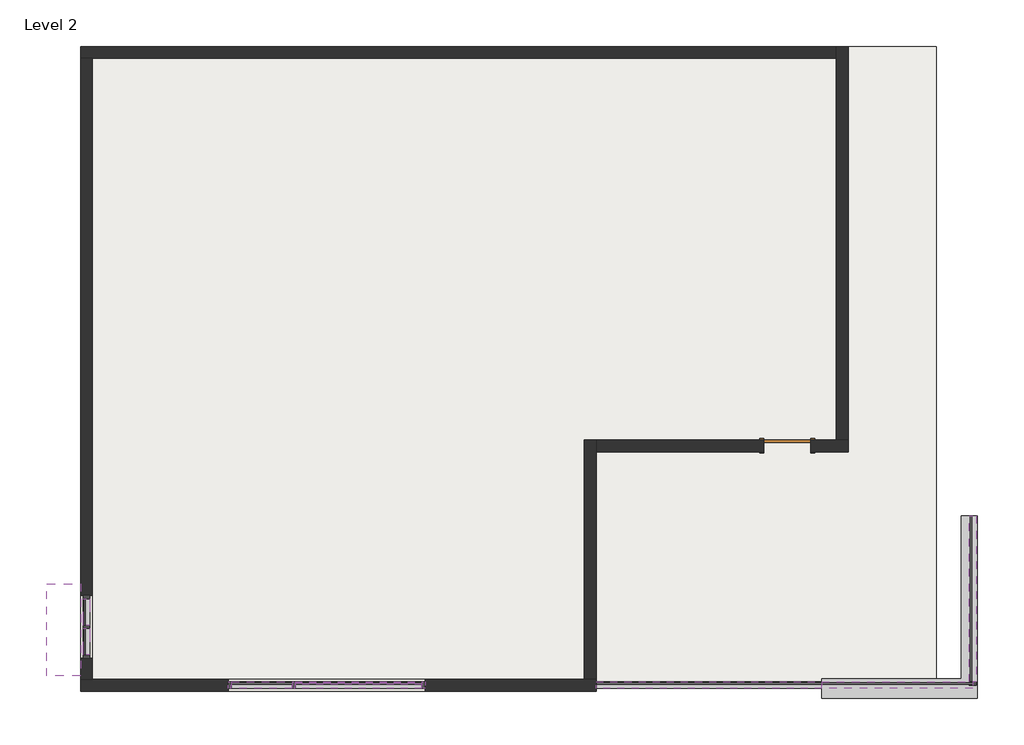
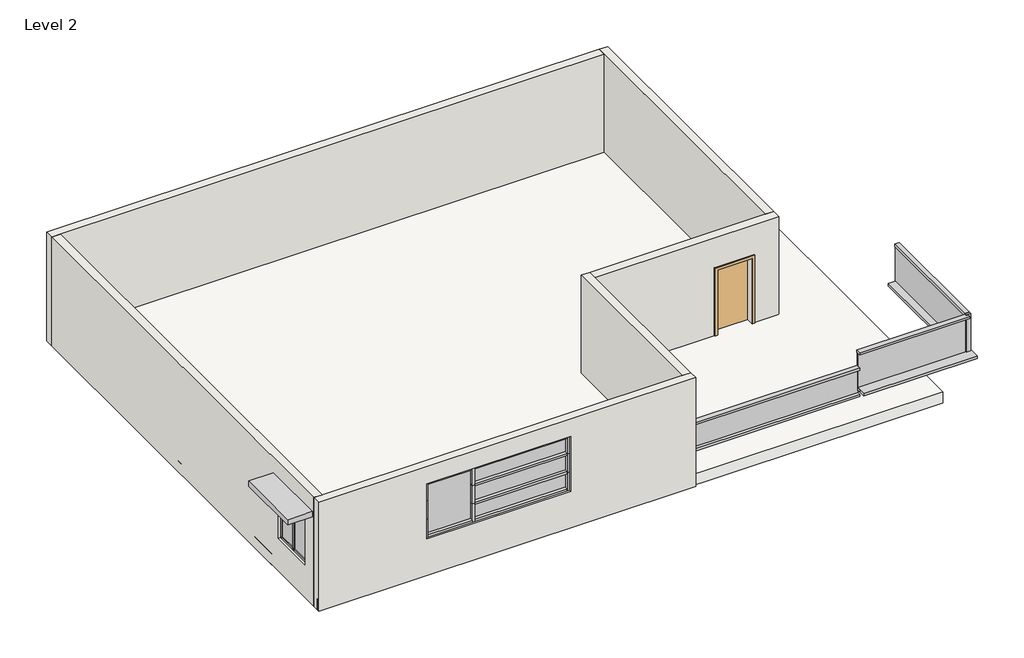
# One storey: 28 members, 9 plates, 6 walls, 2 proxies, 1 door, 1 roof.
"""IFC4 building model written with IfcOpenShell, lengths in millimetres."""

from ifc_helpers import new_model, si_unit, frame, origin, place, context, project, spatial, polyline, outline, extrude, faceted_brep, transform, mapped, element, save
from components import generic_models_3_generic_models_3_8d4ae4f9, generic_models_7_generic_models_7_15f6dc16, door_0ca8825f, member_794f270d, member_fb497cbf, member_38106158, member_c678549b, member_8e6e9988, member_0b7646a3, member_fff16b5b, member_15f14dc2, member_4a27761c, member_d457d5cf, member_01255749, member_1c5922cf, system_panel_glazed_93b0cd61, system_panel_glazed_07248474, system_panel_glazed_5c06d9ac, system_panel_glazed_cb7cf9ed, system_panel_glazed_bff90f26, system_panel_glazed_3fab1137, system_panel_glazed_82fe4a0c

model = new_model("IFC4")

# Units and contexts
model_context = context("Model", 3, world=origin())
ifc_project = project(units=[si_unit("LENGTHUNIT", "METRE", prefix="MILLI")], contexts=[model_context])

# Site, building, storey
site = spatial("IfcSite", under=ifc_project)
building = spatial("IfcBuilding", under=site)
storey = spatial("IfcBuildingStorey", under=building, Name="Level 2", Elevation=3048.0)

# Proxies
placement = place(None, origin())
generic_models_3_generic_models_3_shape = generic_models_3_generic_models_3_8d4ae4f9(model_context)
element("IfcBuildingElementProxy", 1, Name="Generic Models 3 : Generic Models 3", ObjectType="Generic Models 3 : Generic Models 3", at=placement, inside=storey, context=model_context, shape_type="MappedRepresentation", body=[
    mapped(generic_models_3_generic_models_3_shape, transform((0.0, 0.0, 0.0), x_axis=(1.0, 0.0, 0.0), y_axis=(0.0, 1.0, 0.0), z_axis=(0.0, 0.0, 1.0))),
])
generic_models_7_generic_models_7_shape = generic_models_7_generic_models_7_15f6dc16(model_context)
element("IfcBuildingElementProxy", 2, Name="Generic Models 7 : Generic Models 7", ObjectType="Generic Models 7 : Generic Models 7", at=placement, inside=storey, context=model_context, shape_type="MappedRepresentation", body=[
    mapped(generic_models_7_generic_models_7_shape, transform((0.0, 0.0, 0.0), x_axis=(1.0, 0.0, 0.0), y_axis=(0.0, 1.0, 0.0), z_axis=(0.0, 0.0, 1.0))),
])

# Door
door_shape = door_0ca8825f(model_context)
element("IfcDoor", 3, ObjectType="Single-Flush : 36\" x 84\"", at=placement, inside=storey, context=model_context, shape_type="MappedRepresentation", body=[
    mapped(door_shape, transform((-4164.5229687, -6103.4015118, 3048.0), x_axis=(1.0, 0.0, 0.0), y_axis=(0.0, 1.0, 0.0), z_axis=(0.0, 0.0, 1.0))),
])

# Members
member_shape = member_794f270d(model_context)
element("IfcMember", 4, ObjectType="Rectangular Mullion : 2.5\" x 5\" rectangular", at=placement, inside=storey, context=model_context, shape_type="MappedRepresentation", body=[
    mapped(member_shape, transform((-14984.9229687, -10738.9015118, 5099.2464705), x_axis=(-1.0, 0.0, 0.0), y_axis=(0.0, -1.0, 0.0), z_axis=(0.0, 0.0, 1.0))),
])
member_2_shape = member_fb497cbf(model_context)
element("IfcMember", 5, ObjectType="Rectangular Mullion : 2.5\" x 5\" rectangular", at=placement, inside=storey, context=model_context, shape_type="MappedRepresentation", body=[
    mapped(member_2_shape, transform((-14921.4229687, -10738.9015118, 4072.0328571), x_axis=(0.0, 0.0, -1.0), y_axis=(0.0, -1.0, 0.0), z_axis=(-1.0, 0.0, 0.0))),
])
element("IfcMember", 6, ObjectType="Rectangular Mullion : 2.5\" x 5\" rectangular", at=placement, inside=storey, context=model_context, shape_type="MappedRepresentation", body=[
    mapped(member_shape, transform((-14984.9229687, -10738.9015118, 4585.6396638), x_axis=(-1.0, 0.0, 0.0), y_axis=(0.0, -1.0, 0.0), z_axis=(0.0, 0.0, 1.0))),
])
member_3_shape = member_38106158(model_context)
element("IfcMember", 7, ObjectType="Rectangular Mullion : 2.5\" x 5\" rectangular", at=placement, inside=storey, context=model_context, shape_type="MappedRepresentation", body=[
    mapped(member_3_shape, transform((-13714.9229687, -10738.9015118, 4072.0328571), x_axis=(1.0, 0.0, 0.0), y_axis=(0.0, -1.0, 0.0), z_axis=(0.0, 0.0, -1.0))),
])
element("IfcMember", 8, ObjectType="Rectangular Mullion : 2.5\" x 5\" rectangular", at=placement, inside=storey, context=model_context, shape_type="MappedRepresentation", body=[
    mapped(member_3_shape, transform((-13714.9229687, -10738.9015118, 4585.6396638), x_axis=(1.0, 0.0, 0.0), y_axis=(0.0, -1.0, 0.0), z_axis=(0.0, 0.0, -1.0))),
])
element("IfcMember", 9, ObjectType="Rectangular Mullion : 2.5\" x 5\" rectangular", at=placement, inside=storey, context=model_context, shape_type="MappedRepresentation", body=[
    mapped(member_3_shape, transform((-13714.9229687, -10738.9015118, 5099.2464705), x_axis=(1.0, 0.0, 0.0), y_axis=(0.0, -1.0, 0.0), z_axis=(0.0, 0.0, -1.0))),
])
element("IfcMember", 10, ObjectType="Rectangular Mullion : 2.5\" x 5\" rectangular", at=placement, inside=storey, context=model_context, shape_type="MappedRepresentation", body=[
    mapped(member_2_shape, transform((-13746.6729687, -10738.9015118, 5612.8532772), x_axis=(0.0, 0.0, 1.0), y_axis=(0.0, -1.0, 0.0), z_axis=(1.0, 0.0, 0.0))),
])
element("IfcMember", 11, ObjectType="Rectangular Mullion : 2.5\" x 5\" rectangular", at=placement, inside=storey, context=model_context, shape_type="MappedRepresentation", body=[
    mapped(member_shape, transform((-14984.9229687, -10738.9015118, 5612.8532772), x_axis=(-1.0, 0.0, 0.0), y_axis=(0.0, -1.0, 0.0), z_axis=(0.0, 0.0, 1.0))),
])
member_4_shape = member_c678549b(model_context)
element("IfcMember", 12, ObjectType="Rectangular Mullion : 2.5\" x 5\" rectangular", at=placement, inside=storey, context=model_context, shape_type="MappedRepresentation", body=[
    mapped(member_4_shape, transform((-13683.1729687, -10738.9015118, 4072.0328571), x_axis=(0.0, 0.0, -1.0), y_axis=(0.0, -1.0, 0.0), z_axis=(-1.0, 0.0, 0.0))),
])
member_5_shape = member_8e6e9988(model_context)
element("IfcMember", 13, ObjectType="Rectangular Mullion : 2.5\" x 5\" rectangular", at=placement, inside=storey, context=model_context, shape_type="MappedRepresentation", body=[
    mapped(member_5_shape, transform((-11238.4229687, -10738.9015118, 4585.6396638), x_axis=(0.0, 0.0, 1.0), y_axis=(0.0, -1.0, 0.0), z_axis=(1.0, 0.0, 0.0))),
])
element("IfcMember", 14, ObjectType="Rectangular Mullion : 2.5\" x 5\" rectangular", at=placement, inside=storey, context=model_context, shape_type="MappedRepresentation", body=[
    mapped(member_5_shape, transform((-11238.4229687, -10738.9015118, 5099.2464705), x_axis=(0.0, 0.0, 1.0), y_axis=(0.0, -1.0, 0.0), z_axis=(1.0, 0.0, 0.0))),
])
element("IfcMember", 15, ObjectType="Rectangular Mullion : 2.5\" x 5\" rectangular", at=placement, inside=storey, context=model_context, shape_type="MappedRepresentation", body=[
    mapped(member_4_shape, transform((-11238.4229687, -10738.9015118, 5612.8532772), x_axis=(0.0, 0.0, 1.0), y_axis=(0.0, -1.0, 0.0), z_axis=(1.0, 0.0, 0.0))),
])
element("IfcMember", 16, ObjectType="Rectangular Mullion : 2.5\" x 5\" rectangular", at=placement, inside=storey, context=model_context, shape_type="MappedRepresentation", body=[
    mapped(member_shape, transform((-11174.9229687, -10738.9015118, 4585.6396638), x_axis=(1.0, 0.0, 0.0), y_axis=(0.0, -1.0, 0.0), z_axis=(0.0, 0.0, -1.0))),
])
element("IfcMember", 17, ObjectType="Rectangular Mullion : 2.5\" x 5\" rectangular", at=placement, inside=storey, context=model_context, shape_type="MappedRepresentation", body=[
    mapped(member_shape, transform((-11174.9229687, -10738.9015118, 5099.2464705), x_axis=(1.0, 0.0, 0.0), y_axis=(0.0, -1.0, 0.0), z_axis=(0.0, 0.0, -1.0))),
])
element("IfcMember", 18, ObjectType="Rectangular Mullion : 2.5\" x 5\" rectangular", at=placement, inside=storey, context=model_context, shape_type="MappedRepresentation", body=[
    mapped(member_shape, transform((-11174.9229687, -10738.9015118, 4072.0328571), x_axis=(1.0, 0.0, 0.0), y_axis=(0.0, -1.0, 0.0), z_axis=(0.0, 0.0, -1.0))),
])
member_6_shape = member_0b7646a3(model_context)
element("IfcMember", 19, ObjectType="Rectangular Mullion : 2.5\" x 5\" rectangular", at=placement, inside=storey, context=model_context, shape_type="MappedRepresentation", body=[
    mapped(member_6_shape, transform((-17728.1229687, -9576.8515118, 3968.9847878), x_axis=(0.0, 0.0, -1.0), y_axis=(1.0, 0.0, 0.0), z_axis=(0.0, -1.0, 0.0))),
])
element("IfcMember", 20, ObjectType="Rectangular Mullion : 2.5\" x 5\" rectangular", at=placement, inside=storey, context=model_context, shape_type="MappedRepresentation", body=[
    mapped(member_6_shape, transform((-17728.1229687, -10154.7015118, 3968.9847878), x_axis=(0.0, 0.0, -1.0), y_axis=(1.0, 0.0, 0.0), z_axis=(0.0, -1.0, 0.0))),
])
member_7_shape = member_fff16b5b(model_context)
element("IfcMember", 21, ObjectType="Rectangular Mullion : 2.5\" x 5\" rectangular", at=placement, inside=storey, context=model_context, shape_type="MappedRepresentation", body=[
    mapped(member_7_shape, transform((-17728.1229687, -9608.6015118, 3968.9847878), x_axis=(0.0, 1.0, 0.0), y_axis=(1.0, 0.0, 0.0), z_axis=(0.0, 0.0, -1.0))),
])
element("IfcMember", 22, ObjectType="Rectangular Mullion : 2.5\" x 5\" rectangular", at=placement, inside=storey, context=model_context, shape_type="MappedRepresentation", body=[
    mapped(member_6_shape, transform((-17728.1229687, -9640.3515118, 5516.2672692), x_axis=(0.0, 0.0, 1.0), y_axis=(1.0, 0.0, 0.0), z_axis=(0.0, 1.0, 0.0))),
])
element("IfcMember", 23, ObjectType="Rectangular Mullion : 2.5\" x 5\" rectangular", at=placement, inside=storey, context=model_context, shape_type="MappedRepresentation", body=[
    mapped(member_6_shape, transform((-17728.1229687, -9062.5015118, 5516.2672692), x_axis=(0.0, 0.0, 1.0), y_axis=(1.0, 0.0, 0.0), z_axis=(0.0, 1.0, 0.0))),
])
member_8_shape = member_15f14dc2(model_context)
element("IfcMember", 24, ObjectType="Rectangular Mullion : 2.5\" x 5\" rectangular", at=placement, inside=storey, context=model_context, shape_type="MappedRepresentation", body=[
    mapped(member_8_shape, transform((-17728.1229687, -8999.0015118, 3968.9847878), x_axis=(0.0, 1.0, 0.0), y_axis=(1.0, 0.0, 0.0), z_axis=(0.0, 0.0, -1.0))),
])
element("IfcMember", 25, ObjectType="Rectangular Mullion : 2.5\" x 5\" rectangular", at=placement, inside=storey, context=model_context, shape_type="MappedRepresentation", body=[
    mapped(member_8_shape, transform((-17728.1229687, -10218.2015118, 5516.2672692), x_axis=(0.0, -1.0, 0.0), y_axis=(1.0, 0.0, 0.0), z_axis=(0.0, 0.0, 1.0))),
])
member_9_shape = member_4a27761c(model_context)
element("IfcMember", 26, ObjectType="Rectangular Mullion : 2.5\" x 5\" rectangular", at=placement, inside=storey, context=model_context, shape_type="MappedRepresentation", body=[
    mapped(member_9_shape, transform((-3495.9020237, -10738.9015118, 4803.2492128), x_axis=(0.0, 0.0, 1.0), y_axis=(0.0, -1.0, 0.0), z_axis=(1.0, 0.0, 0.0))),
])
element("IfcMember", 27, ObjectType="Rectangular Mullion : 2.5\" x 5\" rectangular", at=placement, inside=storey, context=model_context, shape_type="MappedRepresentation", body=[
    mapped(member_9_shape, transform((-7860.2229687, -10738.9015118, 4005.4438919), x_axis=(0.0, 0.0, -1.0), y_axis=(0.0, -1.0, 0.0), z_axis=(-1.0, 0.0, 0.0))),
])
member_10_shape = member_d457d5cf(model_context)
element("IfcMember", 28, ObjectType="Rectangular Mullion : 2.5\" x 5\" rectangular", at=placement, inside=storey, context=model_context, shape_type="MappedRepresentation", body=[
    mapped(member_10_shape, transform((-574.9020237, -10738.9015118, 5233.9468138), x_axis=(0.0, 0.0, 1.0), y_axis=(0.0, -1.0, 0.0), z_axis=(1.0, 0.0, 0.0))),
])
element("IfcMember", 29, ObjectType="Rectangular Mullion : 2.5\" x 5\" rectangular", at=placement, inside=storey, context=model_context, shape_type="MappedRepresentation", body=[
    mapped(member_10_shape, transform((-3495.9020237, -10738.9015118, 4135.5328571), x_axis=(0.0, 0.0, -1.0), y_axis=(0.0, -1.0, 0.0), z_axis=(-1.0, 0.0, 0.0))),
])
member_11_shape = member_01255749(model_context)
element("IfcMember", 30, ObjectType="Rectangular Mullion : 2.5\" x 5\" rectangular", at=placement, inside=storey, context=model_context, shape_type="MappedRepresentation", body=[
    mapped(member_11_shape, transform((-574.9020237, -7462.3015118, 5252.3696203), x_axis=(0.0, 0.0, 1.0), y_axis=(1.0, 0.0, 0.0), z_axis=(0.0, 1.0, 0.0))),
])
member_12_shape = member_1c5922cf(model_context)
element("IfcMember", 31, ObjectType="Rectangular Mullion : 2.5\" x 5\" rectangular", at=placement, inside=storey, context=model_context, shape_type="MappedRepresentation", body=[
    mapped(member_12_shape, transform((-574.9020237, -10738.9015118, 5252.3696203), x_axis=(0.0, -1.0, 0.0), y_axis=(1.0, 0.0, 0.0), z_axis=(0.0, 0.0, 1.0))),
])

# Plates
system_panel_glazed_shape = system_panel_glazed_93b0cd61(model_context)
element("IfcPlate", 32, ObjectType="System Panel : Glazed", at=placement, inside=storey, context=model_context, shape_type="MappedRepresentation", body=[
    mapped(system_panel_glazed_shape, transform((-14334.0479687, -10738.9015118, 4135.5328571), x_axis=(1.0, 0.0, 0.0), y_axis=(0.0, 1.0, 0.0), z_axis=(0.0, 0.0, 1.0))),
])
system_panel_glazed_2_shape = system_panel_glazed_07248474(model_context)
element("IfcPlate", 33, ObjectType="System Panel : Glazed", at=placement, inside=storey, context=model_context, shape_type="MappedRepresentation", body=[
    mapped(system_panel_glazed_2_shape, transform((-12460.7979687, -10738.9015118, 4135.5328571), x_axis=(1.0, 0.0, 0.0), y_axis=(0.0, 1.0, 0.0), z_axis=(0.0, 0.0, 1.0))),
])
element("IfcPlate", 34, ObjectType="System Panel : Glazed", at=placement, inside=storey, context=model_context, shape_type="MappedRepresentation", body=[
    mapped(system_panel_glazed_2_shape, transform((-12460.7979687, -10738.9015118, 5130.9964705), x_axis=(1.0, 0.0, 0.0), y_axis=(0.0, 1.0, 0.0), z_axis=(0.0, 0.0, 1.0))),
])
system_panel_glazed_3_shape = system_panel_glazed_5c06d9ac(model_context)
element("IfcPlate", 35, ObjectType="System Panel : Glazed", at=placement, inside=storey, context=model_context, shape_type="MappedRepresentation", body=[
    mapped(system_panel_glazed_3_shape, transform((-12460.7979687, -10738.9015118, 4617.3896638), x_axis=(1.0, 0.0, 0.0), y_axis=(0.0, 1.0, 0.0), z_axis=(0.0, 0.0, 1.0))),
])
system_panel_glazed_4_shape = system_panel_glazed_cb7cf9ed(model_context)
element("IfcPlate", 36, ObjectType="System Panel : Glazed", at=placement, inside=storey, context=model_context, shape_type="MappedRepresentation", body=[
    mapped(system_panel_glazed_4_shape, transform((-17728.1229687, -9897.5265118, 4032.4847878), x_axis=(0.0, 1.0, 0.0), y_axis=(-1.0, 0.0, 0.0), z_axis=(0.0, 0.0, 1.0))),
])
element("IfcPlate", 37, ObjectType="System Panel : Glazed", at=placement, inside=storey, context=model_context, shape_type="MappedRepresentation", body=[
    mapped(system_panel_glazed_4_shape, transform((-17728.1229687, -9319.6765118, 4032.4847878), x_axis=(0.0, 1.0, 0.0), y_axis=(-1.0, 0.0, 0.0), z_axis=(0.0, 0.0, 1.0))),
])
system_panel_glazed_5_shape = system_panel_glazed_bff90f26(model_context)
element("IfcPlate", 38, ObjectType="System Panel : Glazed", at=placement, inside=storey, context=model_context, shape_type="MappedRepresentation", body=[
    mapped(system_panel_glazed_5_shape, transform((-5678.0624962, -10738.9015118, 4068.9438919), x_axis=(1.0, 0.0, 0.0), y_axis=(0.0, 1.0, 0.0), z_axis=(0.0, 0.0, 1.0))),
])
system_panel_glazed_6_shape = system_panel_glazed_3fab1137(model_context)
element("IfcPlate", 39, ObjectType="System Panel : Glazed", at=placement, inside=storey, context=model_context, shape_type="MappedRepresentation", body=[
    mapped(system_panel_glazed_6_shape, transform((-2035.4020237, -10738.9015118, 4199.0328571), x_axis=(1.0, 0.0, 0.0), y_axis=(0.0, 1.0, 0.0), z_axis=(0.0, 0.0, 1.0))),
])
system_panel_glazed_7_shape = system_panel_glazed_82fe4a0c(model_context)
element("IfcPlate", 40, ObjectType="System Panel : Glazed", at=placement, inside=storey, context=model_context, shape_type="MappedRepresentation", body=[
    mapped(system_panel_glazed_7_shape, transform((-574.9020237, -9068.8515118, 4135.5328571), x_axis=(0.0, 1.0, 0.0), y_axis=(-1.0, 0.0, 0.0), z_axis=(0.0, 0.0, 1.0))),
])

# Roof
element("IfcRoof", 41, ObjectType="Generic - 12\"", at=placement, inside=storey, context=model_context, shape_type="SweptSolid", body=[
    extrude(outline(polyline([(-17842.4229687, 1630.8984882), (-1278.9002751, 1630.8984882), (-1278.9002751, -10789.7015118), (-17842.4229687, -10789.7015118), (-17842.4229687, 1630.8984882)])), frame((0.0, 0.0, 3048.0), z_axis=(0.0, 0.0, 1.0), x_axis=(1.0, 0.0, 0.0)), (0.0, 0.0, 1.0), 304.8),
])

# Walls
element("IfcWall", 42, ObjectType="9\"", at=placement, inside=storey, context=model_context, shape_type="Brep", body=[
    faceted_brep([(-17842.4229687, -10853.2015118, 3048.0), (-7860.2229687, -10853.2015118, 3048.0), (-7860.2229687, -10853.2015118, 6096.0), (-17842.4229687, -10853.2015118, 6096.0), (-14984.9229687, -10853.2015118, 4072.0328571), (-14984.9229687, -10853.2015118, 5612.8532772), (-11174.9229687, -10853.2015118, 5612.8532772), (-11174.9229687, -10853.2015118, 4072.0328571), (-7860.2229687, -10624.6015118, 3048.0), (-8088.8229687, -10624.6015118, 3048.0), (-17613.8229687, -10624.6015118, 3048.0), (-17842.4229687, -10624.6015118, 3048.0), (-17842.4229687, -10624.6015118, 6096.0), (-17613.8229687, -10624.6015118, 6096.0), (-8088.8229687, -10624.6015118, 6096.0), (-7860.2229687, -10624.6015118, 6096.0), (-14984.9229687, -10624.6015118, 5612.8532772), (-14984.9229687, -10624.6015118, 4072.0328571), (-11174.9229687, -10624.6015118, 4072.0328571), (-11174.9229687, -10624.6015118, 5612.8532772)], [[[0, 1, 2, 3], [4, 5, 6, 7]], [[8, 9, 10, 11, 12, 13, 14, 15], [16, 17, 18, 19]], [[1, 0, 11, 10, 9, 8]], [[3, 2, 15, 14, 13, 12]], [[2, 1, 8, 15]], [[0, 3, 12, 11]], [[4, 17, 16, 5]], [[5, 16, 19, 6]], [[6, 19, 18, 7]], [[17, 4, 7, 18]]]),
])
element("IfcWall", 43, ObjectType="9\"", at=placement, inside=storey, context=model_context, shape_type="Brep", body=[
    faceted_brep([(-7860.2229687, -10624.6015118, 3048.0), (-7860.2229687, -6217.7015118, 3048.0), (-7860.2229687, -5989.1015118, 3048.0), (-7860.2229687, -5989.1015118, 6096.0), (-7860.2229687, -6217.7015118, 6096.0), (-7860.2229687, -10624.6015118, 6096.0), (-8088.8229687, -10624.6015118, 3048.0), (-8088.8229687, -10624.6015118, 6096.0), (-8088.8229687, -5989.1015118, 6096.0), (-8088.8229687, -5989.1015118, 3048.0)], [[[0, 1, 2, 3, 4, 5]], [[6, 7, 8, 9]], [[2, 1, 0, 6, 9]], [[5, 4, 3, 8, 7]], [[0, 5, 7, 6]], [[3, 2, 9, 8]]]),
])
element("IfcWall", 44, ObjectType="9\"", at=placement, inside=storey, context=model_context, shape_type="Brep", body=[
    faceted_brep([(-3707.3229687, -6217.7015118, 5181.6), (-3707.3229687, -6217.7015118, 3048.0), (-2983.4229687, -6217.7015118, 3048.0), (-2983.4229687, -6217.7015118, 6096.0), (-7860.2229687, -6217.7015118, 6096.0), (-7860.2229687, -6217.7015118, 3048.0), (-4621.7229687, -6217.7015118, 3048.0), (-4621.7229687, -6217.7015118, 5181.6), (-2983.4229687, -5989.1015118, 3048.0), (-3212.0229687, -5989.1015118, 3048.0), (-3707.3229687, -5989.1015118, 3048.0), (-3707.3229687, -5989.1015118, 5181.6), (-4621.7229687, -5989.1015118, 5181.6), (-4621.7229687, -5989.1015118, 3048.0), (-7860.2229687, -5989.1015118, 3048.0), (-7860.2229687, -5989.1015118, 6096.0), (-3212.0229687, -5989.1015118, 6096.0), (-2983.4229687, -5989.1015118, 6096.0)], [[[0, 1, 2, 3, 4, 5, 6, 7]], [[8, 9, 10, 11, 12, 13, 14, 15, 16, 17]], [[6, 5, 14, 13]], [[2, 1, 10, 9, 8]], [[4, 3, 17, 16, 15]], [[5, 4, 15, 14]], [[3, 2, 8, 17]], [[11, 10, 1, 0]], [[12, 11, 0, 7]], [[13, 12, 7, 6]]]),
])
element("IfcWall", 45, ObjectType="9\"", at=placement, inside=storey, context=model_context, shape_type="Brep", body=[
    faceted_brep([(-2983.4229687, -5989.1015118, 3048.0), (-2983.4229687, 1630.8984882, 3048.0), (-2983.4229687, 1630.8984882, 6096.0), (-2983.4229687, -5989.1015118, 6096.0), (-3212.0229687, -5989.1015118, 3048.0), (-3212.0229687, -5989.1015118, 6096.0), (-3212.0229687, 1402.2984882, 6096.0), (-3212.0229687, 1630.8984882, 6096.0), (-3212.0229687, 1630.8984882, 3048.0), (-3212.0229687, 1402.2984882, 3048.0)], [[[0, 1, 2, 3]], [[4, 5, 6, 7, 8, 9]], [[1, 0, 4, 9, 8]], [[3, 2, 7, 6, 5]], [[0, 3, 5, 4]], [[2, 1, 8, 7]]]),
])
element("IfcWall", 46, ObjectType="9\"", at=placement, inside=storey, context=model_context, shape_type="Brep", body=[
    faceted_brep([(-3212.0229687, 1630.8984882, 3048.0), (-17842.4229687, 1630.8984882, 3048.0), (-17842.4229687, 1630.8984882, 6096.0), (-3212.0229687, 1630.8984882, 6096.0), (-3212.0229687, 1402.2984882, 3048.0), (-3212.0229687, 1402.2984882, 6096.0), (-17613.8229687, 1402.2984882, 6096.0), (-17842.4229687, 1402.2984882, 6096.0), (-17842.4229687, 1402.2984882, 3048.0), (-17613.8229687, 1402.2984882, 3048.0)], [[[0, 1, 2, 3]], [[4, 5, 6, 7, 8, 9]], [[1, 0, 4, 9, 8]], [[3, 2, 7, 6, 5]], [[0, 3, 5, 4]], [[2, 1, 8, 7]]]),
])
element("IfcWall", 47, ObjectType="9\"", at=placement, inside=storey, context=model_context, shape_type="SweptSolid", body=[
    extrude(outline(polyline([(1402.2984882, 3048.0), (-10624.6015118, 3048.0), (-10624.6015118, 6096.0), (1402.2984882, 6096.0), (1402.2984882, 3048.0)]), holes=[polyline([(-10218.2015118, 5516.2672692), (-10218.2015118, 3968.9847878), (-8999.0015118, 3968.9847878), (-8999.0015118, 5516.2672692), (-10218.2015118, 5516.2672692)])]), frame((-17842.4229687, 0.0, 0.0), z_axis=(1.0, 0.0, 0.0), x_axis=(0.0, 1.0, 0.0)), (0.0, 0.0, 1.0), 228.6),
])

save(model, "model.ifc")

# Revit data of these elements
# Type "Single-Flush : 36\" x 84\""
#   Type Mark = "1"
#   Construction Type Id = "MDOOR"
#   Assembly Code = "C1020"
#   Analytic Construction = "Metal"
#   Thickness = 0' - 2"
#   Heat Transfer Coefficient (U) = 0.651978 BTU/(h·ft²·°F)
#   Height = 7' - 0"
#   Trim Projection Ext = 0' - 1"
#   Trim Projection Int = 0' - 1"
#   Trim Width = 0' - 3"
#   Width = 3' - 0"
#   Define Thermal Properties by = 1
#   Define Thermal Properties by = 1
#   Door Material = Door - Panel
#   Frame Material = Door - Frame
#   Visual Light Transmittance = 0
#   Solar Heat Gain Coefficient = 0
#   Function = (empty or 0)
#   Wall Closure = (empty or 0)
# Type "Rectangular Mullion : 2.5\" x 5\" rectangular"
#   built-in parameter 1007304 = 0.416667 (stored number, unit not read)
#   built-in parameter 1007301 = 0.104167 (stored number, unit not read)
#   built-in parameter 1007300 = 0.104167 (stored number, unit not read)
# Type "System Panel : Glazed"
#   Construction Type Id = "GSP4R"
#   Analytic Construction = "1/8 in Pilkington single glazing"
#   Visual Light Transmittance = 0.9
#   Solar Heat Gain Coefficient = 0.86
#   Heat Transfer Coefficient (U) = 1.18115 BTU/(h·ft²·°F)
#   Define Thermal Properties by = 1
# Type "Generic - 12\""
#   Assembly Code = "B1020"
#   Layers, outside or top first: 1' - 0" no material (function 1)
# Type "9\""
#   Assembly Code = "B2010"
#   Layers, outside or top first: 0' - 9" no material (function 1)
# Element 1 (IfcBuildingElementProxy, "Generic Models 3 : Generic Models 3")
#   Phase Created = New Construction
# Element 2 (IfcBuildingElementProxy, "Generic Models 7 : Generic Models 7")
#   Phase Created = New Construction
# Element 3 (IfcDoor, "Single-Flush : 36\" x 84\"")
#   Phase Created = New Construction
#   Materials on its faces: "Door - Frame", "Door - Panel"
# Elements 4, 5, 6, 7, 8, 9, 10, 11, 12, 13, 14, 15, 16, 17, 18, 19, 20, 21, 22, 23, 24, 25, 26, 27, 28, 29, 30, 31 (IfcMember, "Rectangular Mullion : 2.5\" x 5\" rectangular")
#   Phase Created = New Construction
#   Materials on its faces: "Aluminum"
# Elements 32, 33, 34, 35, 36, 37, 38, 39, 40 (IfcPlate, "System Panel : Glazed")
#   Phase Created = New Construction
#   Materials on its faces: "Glass"
# Element 41 (IfcRoof, "Generic - 12\"")
#   built-in parameter 1001705 = 11 (stored number, unit not read)
#   built-in parameter 1001710 = 33615
#   Phase Created = New Construction
#   Materials on its faces: "Default Roof"
# Elements 42, 43, 44, 45, 46, 47 (IfcWall, "9\"")
#   Top Offset = 0' - 0"
#   Base Offset = 0' - 0"
#   Unconnected Height = 10' - 0"
#   wall height = 10' - 0"
#   Phase Created = New Construction
#   Base Constraint = Level 2
#   Materials on its faces: "Default Wall"
# Materials
#   "Door - Panel": class "Wood", colour RGB 210 159 95, transparency 0, Cost = 0
#   "Door - Frame": colour RGB 118 70 51, transparency 0, Cost = 0
#   "Aluminum": class "Metal", colour RGB 247 247 247, transparency 0, Description = "Aluminum 6061", Cost = 0
#   "Glass": class "Glass", colour RGB 0 128 192, transparency 0.75, Description = "Soda Lime Glass", Cost = 0
#   "Default Roof": colour RGB 88 101 114, transparency 0, Cost = 0
#   "Default Wall": colour RGB 128 128 128, transparency 0, Cost = 0
